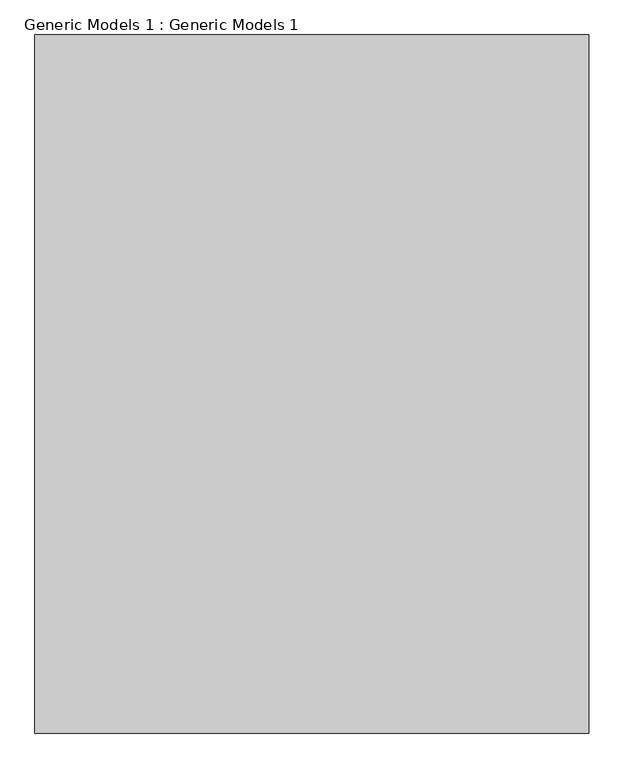
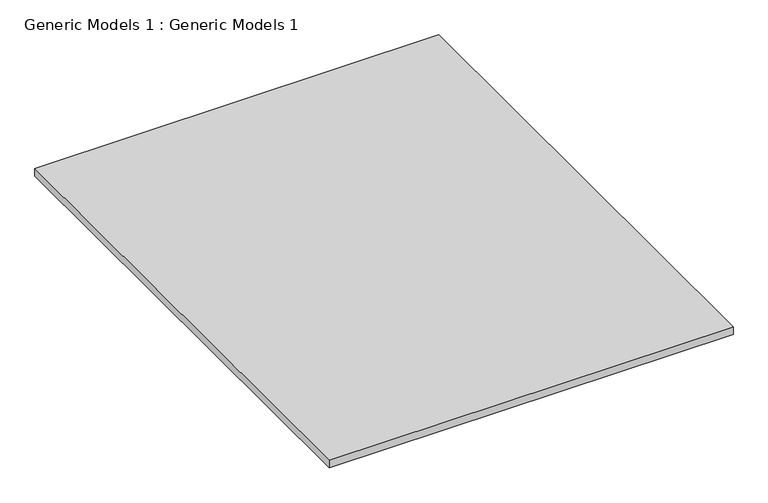
"""IFC4 building model written with IfcOpenShell, lengths in millimetres: proxy geometry, Generic Models 1 : Generic Models 1."""

from ifc_helpers import new_model, si_unit, frame, origin, place, context, project, spatial, polyline, outline, extrude, source, transform, mapped, element, save


def generic_models_1_generic_models_1_a3900748(model_context):
    return source(origin(), model_context, "Body", "SweptSolid", [
        extrude(outline(polyline([(-6669.6094994, 2512.5006048), (-6669.6094994, -17258.2805842), (-22349.7112937, -17258.2805842), (-22349.7112937, 2512.5006048), (-6669.6094994, 2512.5006048)])), frame((0.0, 0.0, -304.8), z_axis=(0.0, 0.0, 1.0), x_axis=(1.0, 0.0, 0.0)), (0.0, 0.0, 1.0), 304.8),
    ])


if __name__ == "__main__":
    model = new_model("IFC4")
    model_context = context("Model", 3, world=origin())
    ifc_project = project(units=[si_unit("LENGTHUNIT", "METRE", prefix="MILLI")], contexts=[model_context])
    site = spatial("IfcSite", under=ifc_project)
    building = spatial("IfcBuilding", under=site)
    placement = place(None, origin())
    generic_models_1_generic_models_1_shape = generic_models_1_generic_models_1_a3900748(model_context)
    element("IfcBuildingElementProxy", 1, Name="Generic Models 1 : Generic Models 1", ObjectType="Generic Models 1 : Generic Models 1", at=placement, inside=building, context=model_context, shape_type="MappedRepresentation", body=[
        mapped(generic_models_1_generic_models_1_shape, transform((0.0, 0.0, 0.0), x_axis=(1.0, 0.0, 0.0), y_axis=(0.0, 1.0, 0.0), z_axis=(0.0, 0.0, 1.0))),
    ])
    save(model, "model.ifc")
